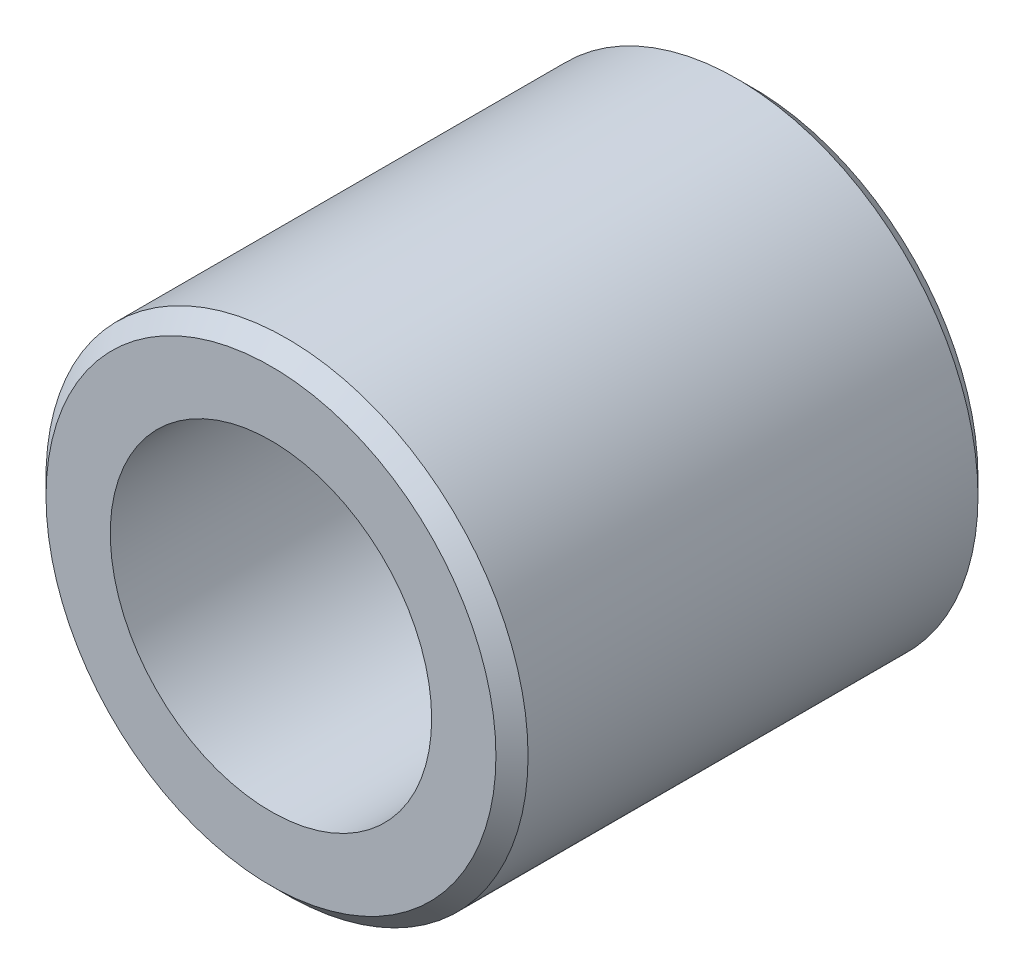
from build123d import *

# Parameters (mm, degrees)
BUSHING_PROFILE_30_20_R       = 15
BUSHING_PROFILE_30_20_R_2     = 10
BUSHING_BODY_L30_DEPTH        = 15
OUTER_EDGE_CHAMFERS_1X45_SIZE = 1


with BuildPart() as part:
    # Bushing Profile Ø30-Ø20 → Bushing Body L30 (new, symmetric)
    with BuildSketch(Plane.XY):
        Circle(BUSHING_PROFILE_30_20_R)
        Circle(BUSHING_PROFILE_30_20_R_2, mode=Mode.SUBTRACT)
    extrude(amount=BUSHING_BODY_L30_DEPTH, both=True)

    # Outer Edge Chamfers 1x45°
    outer_edge_chamfers_1x45_edges = [part.edges().sort_by_distance(p)[0] for p in [
        (-15, 0, -15),
        (-15, 0, 15),
    ]]
    chamfer(outer_edge_chamfers_1x45_edges, length=OUTER_EDGE_CHAMFERS_1X45_SIZE)


solid = part.part
